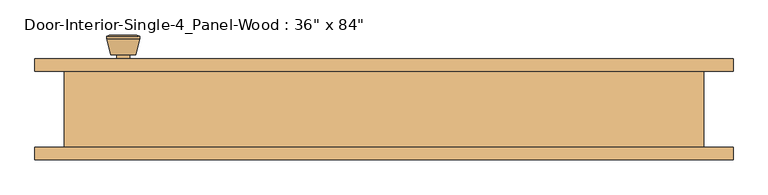
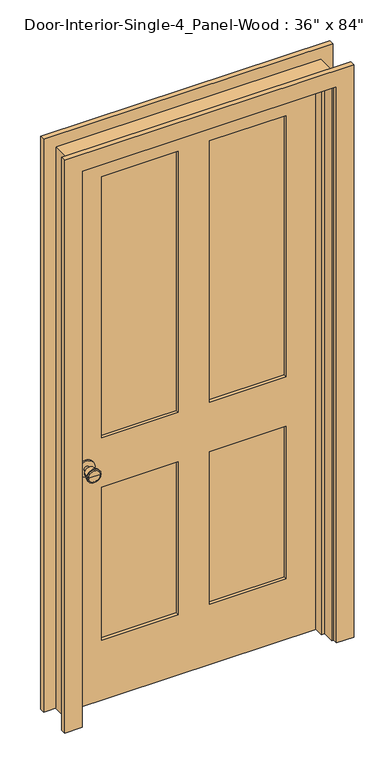
"""IFC4 building model written with IfcOpenShell, lengths in millimetres: door geometry."""

from ifc_helpers import new_model, si_unit, point, frame, frame_2d, origin, place, context, project, spatial, polyline, circle_curve, trimmed, segment, composite_curve, outline, extrude, faceted_brep, source, transform, mapped, element, save
from ifc_brep_helpers import plane_surface, cylinder_surface, revolved_surface, advanced_brep


def door_c2926031(model_context):
    return source(origin(), model_context, "Body", "SolidModel", [
        advanced_brep(
        [(-393.7, 13.05, 914.4), (-383.7, 13.05, 914.4), (-403.7, 13.05, 914.4), (-373.2241324, -35.95, 914.4), (-393.7, -35.95, 914.4), (-414.1758676, -35.95, 914.4), (-368.7, -34.1221319, 914.4), (-418.7, -34.1221319, 914.4), (-368.7, -30.6584537, 914.4), (-418.7, -30.6584537, 914.4), (-375.063764, -5.95, 914.4), (-412.336236, -5.95, 914.4), (-383.7, -5.95, 914.4), (-403.7, -5.95, 914.4)],
        [
            (0, 1),
            (1, 2, circle_curve(frame((-393.7, 13.05, 914.4), z_axis=(0.0, 1.0, 0.0), x_axis=(-1.0, 0.0, 0.0)), 10.0)),
            (2, 0),
            (2, 1, circle_curve(frame((-393.7, 13.05, 914.4), z_axis=(0.0, 1.0, 0.0), x_axis=(-1.0, 0.0, 0.0)), 10.0)),
            (3, 4),
            (4, 5),
            (5, 3, circle_curve(frame((-393.7, -35.95, 914.4), z_axis=(0.0, -1.0, 0.0), x_axis=(-1.0, 0.0, 0.0)), 20.4758676)),
            (3, 5, circle_curve(frame((-393.7, -35.95, 914.4), z_axis=(0.0, -1.0, 0.0), x_axis=(-1.0, 0.0, 0.0)), 20.4758676)),
            (6, 3),
            (5, 7),
            (7, 6, circle_curve(frame((-393.7, -34.1221319, 914.4), z_axis=(0.0, -1.0, 0.0), x_axis=(-1.0, 0.0, 0.0)), 25.0)),
            (6, 7, circle_curve(frame((-393.7, -34.1221319, 914.4), z_axis=(0.0, -1.0, 0.0), x_axis=(-1.0, 0.0, 0.0)), 25.0)),
            (8, 6),
            (7, 9),
            (9, 8, circle_curve(frame((-393.7, -30.6584537, 914.4), z_axis=(0.0, -1.0, 0.0), x_axis=(-1.0, 0.0, 0.0)), 25.0)),
            (8, 9, circle_curve(frame((-393.7, -30.6584537, 914.4), z_axis=(0.0, -1.0, 0.0), x_axis=(-1.0, 0.0, 0.0)), 25.0)),
            (10, 8),
            (9, 11),
            (11, 10, circle_curve(frame((-393.7, -5.95, 914.4), z_axis=(0.0, -1.0, 0.0), x_axis=(-1.0, 0.0, 0.0)), 18.636236)),
            (10, 11, circle_curve(frame((-393.7, -5.95, 914.4), z_axis=(0.0, -1.0, 0.0), x_axis=(-1.0, 0.0, 0.0)), 18.636236)),
            (12, 10),
            (11, 13),
            (13, 12, circle_curve(frame((-393.7, -5.95, 914.4), z_axis=(0.0, -1.0, 0.0), x_axis=(-1.0, 0.0, 0.0)), 10.0)),
            (12, 13, circle_curve(frame((-393.7, -5.95, 914.4), z_axis=(0.0, -1.0, 0.0), x_axis=(-1.0, 0.0, 0.0)), 10.0)),
            (1, 12),
            (13, 2),
        ],
        [
            plane_surface(frame((-393.7, 13.05, 914.4), z_axis=(0.0, 1.0, 0.0), x_axis=(-1.0, 0.0, 0.0))),
            plane_surface(frame((-393.7, -35.95, 914.4), z_axis=(0.0, -1.0, 0.0), x_axis=(-1.0, 0.0, 0.0))),
            revolved_surface(polyline([(-414.1758676, -35.95, 914.4), (-418.7, -34.1221319, 914.4)]), (-393.7, 13.05, 914.4), (0.0, 1.0, 0.0)),
            cylinder_surface(frame((-393.7, 13.05, 914.4), z_axis=(0.0, 1.0, 0.0), x_axis=(-1.0, 0.0, 0.0)), 25.0),
            revolved_surface(polyline([(-418.7, -30.6584537, 914.4), (-412.336236, -5.95, 914.4)]), (-393.7, 13.05, 914.4), (0.0, 1.0, 0.0)),
            plane_surface(frame((-393.7, -5.95, 914.4), z_axis=(0.0, 1.0, 0.0), x_axis=(-1.0, 0.0, 0.0))),
            cylinder_surface(frame((-393.7, 13.05, 914.4), z_axis=(0.0, 1.0, 0.0), x_axis=(-1.0, 0.0, 0.0)), 10.0),
        ],
        [
            (0, [[1, 2, 3]]),
            (0, [[-3, 4, -1]]),
            (1, [[5, 6, 7]]),
            (1, [[-6, -5, 8]]),
            (2, [[9, -7, 10, 11]]),
            (2, [[-10, -8, -9, 12]]),
            (3, [[13, -11, 14, 15]]),
            (3, [[-14, -12, -13, 16]]),
            (4, [[17, -15, 18, 19]]),
            (4, [[-18, -16, -17, 20]]),
            (5, [[21, -19, 22, 23]]),
            (5, [[-22, -20, -21, 24]]),
            (6, [[25, -23, 26, -2]]),
            (6, [[-26, -24, -25, -4]]),
        ],
    ),
        extrude(outline(composite_curve([segment(trimmed(circle_curve(frame_2d((914.4, -393.7)), 30.0), [point((914.4, -423.7))], [point((914.4, -363.7))], False, "CARTESIAN"), True, "CONTINUOUS"), segment(trimmed(circle_curve(frame_2d((914.4, -393.7)), 30.0), [point((914.4, -363.7))], [point((914.4, -423.7))], False, "CARTESIAN"), True, "CONTINUOUS")], self_intersect=False)), frame((0.0, 13.05, 0.0), z_axis=(0.0, 1.0, 0.0), x_axis=(0.0, 0.0, 1.0)), (0.0, 0.0, 1.0), 6.0),
        advanced_brep(
        [(-393.7, 59.975, 914.4), (-403.7, 59.975, 914.4), (-383.7, 59.975, 914.4), (-373.2241324, 108.975, 914.4), (-414.1758676, 108.975, 914.4), (-393.7, 108.975, 914.4), (-368.7, 107.1471319, 914.4), (-418.7, 107.1471319, 914.4), (-368.7, 103.6834537, 914.4), (-418.7, 103.6834537, 914.4), (-375.063764, 78.975, 914.4), (-412.336236, 78.975, 914.4), (-383.7, 78.975, 914.4), (-403.7, 78.975, 914.4)],
        [
            (0, 1),
            (1, 2, circle_curve(frame((-393.7, 59.975, 914.4), z_axis=(0.0, -1.0, 0.0), x_axis=(-1.0, 0.0, 0.0)), 10.0)),
            (2, 0),
            (2, 1, circle_curve(frame((-393.7, 59.975, 914.4), z_axis=(0.0, -1.0, 0.0), x_axis=(-1.0, 0.0, 0.0)), 10.0)),
            (3, 4, circle_curve(frame((-393.7, 108.975, 914.4), z_axis=(0.0, 1.0, 0.0), x_axis=(-1.0, 0.0, 0.0)), 20.4758676)),
            (4, 5),
            (5, 3),
            (4, 3, circle_curve(frame((-393.7, 108.975, 914.4), z_axis=(0.0, 1.0, 0.0), x_axis=(-1.0, 0.0, 0.0)), 20.4758676)),
            (6, 7, circle_curve(frame((-393.7, 107.1471319, 914.4), z_axis=(0.0, 1.0, 0.0), x_axis=(-1.0, 0.0, 0.0)), 25.0)),
            (7, 4),
            (3, 6),
            (7, 6, circle_curve(frame((-393.7, 107.1471319, 914.4), z_axis=(0.0, 1.0, 0.0), x_axis=(-1.0, 0.0, 0.0)), 25.0)),
            (8, 9, circle_curve(frame((-393.7, 103.6834537, 914.4), z_axis=(0.0, 1.0, 0.0), x_axis=(-1.0, 0.0, 0.0)), 25.0)),
            (9, 7),
            (6, 8),
            (9, 8, circle_curve(frame((-393.7, 103.6834537, 914.4), z_axis=(0.0, 1.0, 0.0), x_axis=(-1.0, 0.0, 0.0)), 25.0)),
            (10, 11, circle_curve(frame((-393.7, 78.975, 914.4), z_axis=(0.0, 1.0, 0.0), x_axis=(-1.0, 0.0, 0.0)), 18.636236)),
            (11, 9),
            (8, 10),
            (11, 10, circle_curve(frame((-393.7, 78.975, 914.4), z_axis=(0.0, 1.0, 0.0), x_axis=(-1.0, 0.0, 0.0)), 18.636236)),
            (12, 13, circle_curve(frame((-393.7, 78.975, 914.4), z_axis=(0.0, 1.0, 0.0), x_axis=(-1.0, 0.0, 0.0)), 10.0)),
            (13, 11),
            (10, 12),
            (13, 12, circle_curve(frame((-393.7, 78.975, 914.4), z_axis=(0.0, 1.0, 0.0), x_axis=(-1.0, 0.0, 0.0)), 10.0)),
            (1, 13),
            (12, 2),
        ],
        [
            plane_surface(frame((-393.7, 59.975, 914.4), z_axis=(0.0, -1.0, 0.0), x_axis=(-1.0, 0.0, 0.0))),
            plane_surface(frame((-393.7, 108.975, 914.4), z_axis=(0.0, 1.0, 0.0), x_axis=(-1.0, 0.0, 0.0))),
            revolved_surface(polyline([(-414.1758676, 108.975, 914.4), (-418.7, 107.1471319, 914.4)]), (-393.7, 59.975, 914.4), (0.0, -1.0, 0.0)),
            cylinder_surface(frame((-393.7, 59.975, 914.4), z_axis=(0.0, -1.0, 0.0), x_axis=(-1.0, 0.0, 0.0)), 25.0),
            revolved_surface(polyline([(-418.7, 103.6834537, 914.4), (-412.336236, 78.975, 914.4)]), (-393.7, 59.975, 914.4), (0.0, -1.0, 0.0)),
            plane_surface(frame((-393.7, 78.975, 914.4), z_axis=(0.0, -1.0, 0.0), x_axis=(-1.0, 0.0, 0.0))),
            cylinder_surface(frame((-393.7, 59.975, 914.4), z_axis=(0.0, -1.0, 0.0), x_axis=(-1.0, 0.0, 0.0)), 10.0),
        ],
        [
            (0, [[1, 2, 3]]),
            (0, [[-3, 4, -1]]),
            (1, [[5, 6, 7]]),
            (1, [[8, -7, -6]]),
            (2, [[9, 10, -5, 11]]),
            (2, [[12, -11, -8, -10]]),
            (3, [[13, 14, -9, 15]]),
            (3, [[16, -15, -12, -14]]),
            (4, [[17, 18, -13, 19]]),
            (4, [[20, -19, -16, -18]]),
            (5, [[21, 22, -17, 23]]),
            (5, [[24, -23, -20, -22]]),
            (6, [[-2, 25, -21, 26]]),
            (6, [[-4, -26, -24, -25]]),
        ],
    ),
        extrude(outline(composite_curve([segment(trimmed(circle_curve(frame_2d((914.4, -393.7)), 30.0), [point((914.4, -423.7))], [point((914.4, -363.7))], False, "CARTESIAN"), True, "CONTINUOUS"), segment(trimmed(circle_curve(frame_2d((914.4, -393.7)), 30.0), [point((914.4, -363.7))], [point((914.4, -423.7))], False, "CARTESIAN"), True, "CONTINUOUS")], self_intersect=False)), frame((0.0, 53.975, 0.0), z_axis=(0.0, 1.0, 0.0), x_axis=(0.0, 0.0, 1.0)), (0.0, 0.0, 1.0), 6.0),
        faceted_brep([(482.6, 53.975, 0.0), (482.6, -60.325, 0.0), (457.2, -60.325, 0.0), (457.2, -15.875, 0.0), (444.5, -15.875, 0.0), (444.5, 19.05, 0.0), (457.2, 19.05, 0.0), (457.2, 53.975, 0.0), (482.6, 53.975, 2159.0), (482.6, -60.325, 2159.0), (-482.6, -60.325, 2159.0), (-482.6, -60.325, 0.0), (-457.2, -60.325, 0.0), (-457.2, -60.325, 2133.6), (457.2, -60.325, 2133.6), (457.2, -15.875, 2133.6), (-457.2, -15.875, 2133.6), (-457.2, -15.875, 0.0), (-444.5, -15.875, 0.0), (-444.5, -15.875, 2120.9), (444.5, -15.875, 2120.9), (444.5, 19.05, 2120.9), (-444.5, 19.05, 2120.9), (-444.5, 19.05, 0.0), (-457.2, 19.05, 0.0), (-457.2, 19.05, 2133.6), (457.2, 19.05, 2133.6), (457.2, 53.975, 2133.6), (-457.2, 53.975, 2133.6), (-457.2, 53.975, 0.0), (-482.6, 53.975, 0.0), (-482.6, 53.975, 2159.0)], [[[0, 1, 2, 3, 4, 5, 6, 7]], [[1, 0, 8, 9]], [[2, 1, 9, 10, 11, 12, 13, 14]], [[3, 2, 14, 15]], [[4, 3, 15, 16, 17, 18, 19, 20]], [[5, 4, 20, 21]], [[6, 5, 21, 22, 23, 24, 25, 26]], [[7, 6, 26, 27]], [[0, 7, 27, 28, 29, 30, 31, 8]], [[9, 8, 31, 10]], [[15, 14, 13, 16]], [[21, 20, 19, 22]], [[27, 26, 25, 28]], [[30, 29, 24, 23, 18, 17, 12, 11]], [[10, 31, 30, 11]], [[16, 13, 12, 17]], [[22, 19, 18, 23]], [[28, 25, 24, 29]]]),
        extrude(outline(polyline([(2133.6, -457.2), (0.0, -457.2), (0.0, 457.2), (2133.6, 457.2), (2133.6, -457.2)]), holes=[polyline([(2014.5375, 57.15), (2014.5375, 336.55), (1009.65, 336.55), (1009.65, 57.15), (2014.5375, 57.15)]), polyline([(1009.65, -57.15), (1009.65, -336.55), (2014.5375, -336.55), (2014.5375, -57.15), (1009.65, -57.15)]), polyline([(819.15, 57.15), (819.15, 336.55), (231.775, 336.55), (231.775, 57.15), (819.15, 57.15)]), polyline([(231.775, -57.15), (231.775, -336.55), (819.15, -336.55), (819.15, -57.15), (231.775, -57.15)])]), frame((0.0, 19.05, 0.0), z_axis=(0.0, 1.0, 0.0), x_axis=(0.0, 0.0, 1.0)), (0.0, 0.0, 1.0), 34.925),
        extrude(outline(polyline([(336.55, 30.6916667), (57.15, 30.6916667), (57.15, 42.3333333), (336.55, 42.3333333), (336.55, 30.6916667)])), frame((0.0, 0.0, 1009.65), z_axis=(0.0, 0.0, 1.0), x_axis=(1.0, 0.0, 0.0)), (0.0, 0.0, 1.0), 1004.8875),
        extrude(outline(polyline([(-57.15, 30.6916667), (-336.55, 30.6916667), (-336.55, 42.3333333), (-57.15, 42.3333333), (-57.15, 30.6916667)])), frame((0.0, 0.0, 1009.65), z_axis=(0.0, 0.0, 1.0), x_axis=(1.0, 0.0, 0.0)), (0.0, 0.0, 1.0), 1004.8875),
        extrude(outline(polyline([(336.55, 30.6916667), (57.15, 30.6916667), (57.15, 42.3333333), (336.55, 42.3333333), (336.55, 30.6916667)])), frame((0.0, 0.0, 231.775), z_axis=(0.0, 0.0, 1.0), x_axis=(1.0, 0.0, 0.0)), (0.0, 0.0, 1.0), 587.375),
        extrude(outline(polyline([(-57.15, 30.6916667), (-336.55, 30.6916667), (-336.55, 42.3333333), (-57.15, 42.3333333), (-57.15, 30.6916667)])), frame((0.0, 0.0, 231.775), z_axis=(0.0, 0.0, 1.0), x_axis=(1.0, 0.0, 0.0)), (0.0, 0.0, 1.0), 587.375),
        extrude(outline(polyline([(0.0, 463.55), (0.0, 527.05), (2203.45, 527.05), (2203.45, -527.05), (0.0, -527.05), (0.0, -463.55), (2139.95, -463.55), (2139.95, 463.55), (0.0, 463.55)])), frame((0.0, 53.975, 0.0), z_axis=(0.0, 1.0, 0.0), x_axis=(0.0, 0.0, 1.0)), (0.0, 0.0, 1.0), 19.05),
        extrude(outline(polyline([(0.0, 463.55), (0.0, 527.05), (2203.45, 527.05), (2203.45, -527.05), (0.0, -527.05), (0.0, -463.55), (2139.95, -463.55), (2139.95, 463.55), (0.0, 463.55)])), frame((0.0, -79.375, 0.0), z_axis=(0.0, 1.0, 0.0), x_axis=(0.0, 0.0, 1.0)), (0.0, 0.0, 1.0), 19.05),
    ])


if __name__ == "__main__":
    model = new_model("IFC4")
    model_context = context("Model", 3, world=origin())
    ifc_project = project(units=[si_unit("LENGTHUNIT", "METRE", prefix="MILLI")], contexts=[model_context])
    site = spatial("IfcSite", under=ifc_project)
    building = spatial("IfcBuilding", under=site)
    placement = place(None, origin())
    door_shape = door_c2926031(model_context)
    element("IfcDoor", 1, ObjectType="Door-Interior-Single-4_Panel-Wood : 36\" x 84\"", at=placement, inside=building, context=model_context, shape_type="MappedRepresentation", body=[
        mapped(door_shape, transform((0.0, 0.0, 0.0), x_axis=(1.0, 0.0, 0.0), y_axis=(0.0, 1.0, 0.0), z_axis=(0.0, 0.0, 1.0))),
    ])
    save(model, "model.ifc")

# Revit data of these elements
# Type "Door-Interior-Single-4_Panel-Wood : 36\" x 84\""
#   Type Mark = "10"
#   Assembly Code = "C1020300"
#   Analytic Construction = "Wooden"
#   Top Rail = 0' - 4 11/16"
#   Thickness = 0' - 1 3/8"
#   Thermal Resistance (R) = 2.5876 (h·ft²·°F)/BTU
#   Swing Angle [instance default] = 90.00°
#   Stiles = 0' - 4 3/4"
#   Rough Width = 3' - 2"
#   Rough Height = 7' - 1"
#   Mullion = 0' - 4 1/2"
#   Lock Rail = 0' - 7 1/2"
#   Height = 7' - 0"
#   Width = 3' - 0"
#   Heat Transfer Coefficient (U) = 0.3865 BTU/(h·ft²·°F)
#   Bottom Rail = 0' - 9 1/8"
#   Trim Material = Cherry
#   Panel Material = Cherry
#   Frame Material = Cherry
#   Door Handle Material = Aluminum
#   Visual Light Transmittance = 0
#   Solar Heat Gain Coefficient = 0
#   Wall Closure = (empty or 0)
#   Function = (empty or 0)
# Element 1 (IfcDoor, "Door-Interior-Single-4_Panel-Wood : 36\" x 84\"")
#   Materials on its faces: "Cherry", "Aluminum"
# Materials
#   "Cherry": class "Wood", colour RGB 226 177 128, transparency 0, Description = "Prunus Serotina", Cost = 0
#   "Aluminum": class "Metal", colour RGB 247 247 247, transparency 0, Description = "Aluminum 6061", Cost = 0
